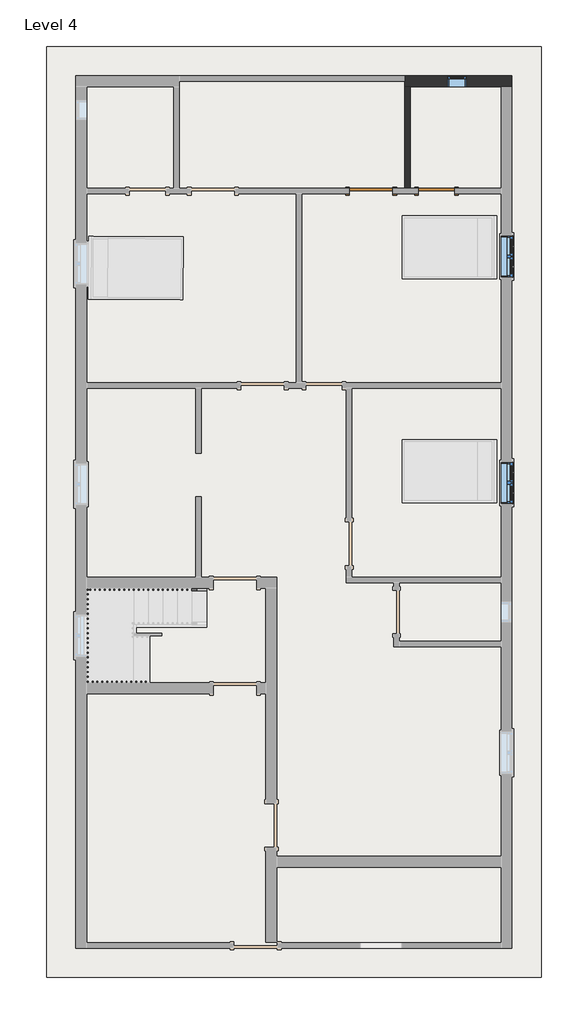
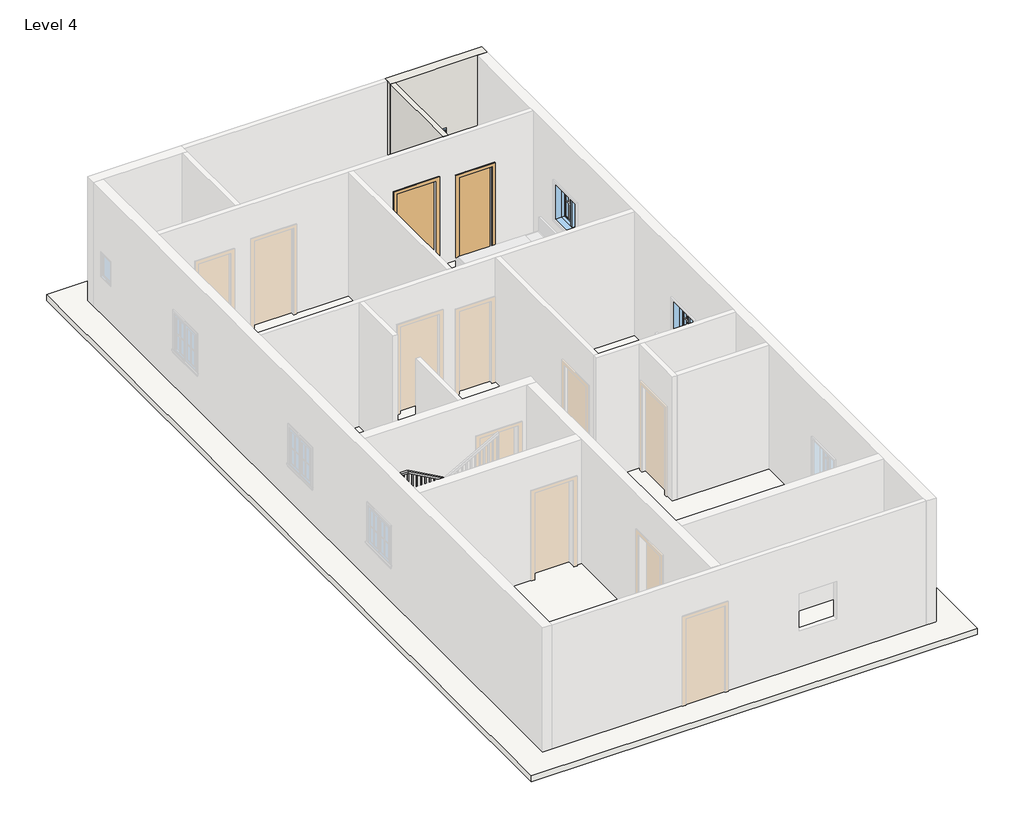
# One storey, part 2 of 3: 3 windows, 2 doors, 2 walls, 1 railing, 1 roof.
"""IFC4 building model written with IfcOpenShell, lengths in millimetres."""

from ifc_helpers import new_model, si_unit, frame, origin, place, context, project, spatial, polyline, outline, extrude, faceted_brep, transform, mapped, element, save
from components import door_f2b275c1, door_e5f9f3c4, window_aa618e30, window_339605e1

model = new_model("IFC4")

# Units and contexts
model_context = context("Model", 3, world=origin())
ifc_project = project(units=[si_unit("LENGTHUNIT", "METRE", prefix="MILLI")], contexts=[model_context])

# Site, building, storey
site = spatial("IfcSite", under=ifc_project)
building = spatial("IfcBuilding", under=site)
storey = spatial("IfcBuildingStorey", under=building, Name="Level 4", Elevation=6400.8)

# Doors
placement = place(None, origin())
door_shape = door_f2b275c1(model_context)
element("IfcDoor", 1, ObjectType="Single-Flush : 30\" x 80\"", at=placement, inside=storey, context=model_context, shape_type="MappedRepresentation", body=[
    mapped(door_shape, transform((1735.6084916, 8007.7072267, 6400.8), x_axis=(-1.0, 0.0, 0.0), y_axis=(0.0, -1.0, 0.0), z_axis=(0.0, 0.0, 1.0))),
])
door_2_shape = door_e5f9f3c4(model_context)
element("IfcDoor", 2, ObjectType="Single-Flush : 36\" x 84\"", at=placement, inside=storey, context=model_context, shape_type="MappedRepresentation", body=[
    mapped(door_2_shape, transform((364.0084916, 8007.7072267, 6400.8), x_axis=(1.0, 0.0, 0.0), y_axis=(0.0, 1.0, 0.0), z_axis=(0.0, 0.0, 1.0))),
])

# Railing
element("IfcRailing", 3, ObjectType="Handrail - Rectangular", at=placement, inside=storey, context=model_context, shape_type="SolidModel", body=[
    faceted_brep([(-3084.0415084, -367.9427733, 7484.5333333), (-3084.0415084, -367.9427733, 7426.420221), (-3084.0415084, -317.1427733, 7426.420221), (-3084.0415084, -317.1427733, 7484.5333333), (-4608.0415084, -367.9427733, 8331.2), (-4621.2051106, -367.9427733, 8280.4), (-4621.2051106, -317.1427733, 8280.4), (-4608.0415084, -317.1427733, 8331.2), (-5547.8415084, -367.9427733, 8331.2), (-5547.8415084, -367.9427733, 8280.4), (-5598.6415084, -317.1427733, 8280.4), (-5598.6415084, -317.1427733, 8331.2), (-5547.8415084, -2247.5427733, 8331.2), (-5547.8415084, -2247.5427733, 8280.4), (-5598.6415084, -2298.3427733, 8280.4), (-5598.6415084, -2298.3427733, 8331.2), (-4912.8415084, -2247.5427733, 8331.2), (-4899.6779062, -2247.5427733, 8280.4), (-4899.6779062, -2298.3427733, 8280.4), (-4912.8415084, -2298.3427733, 8331.2), (-3084.0415084, -2247.5427733, 9347.2), (-3084.0415084, -2298.3427733, 9347.2), (-3084.0415084, -2298.3427733, 9289.0868876), (-3084.0415084, -2247.5427733, 9289.0868876)], [[[0, 1, 2, 3]], [[1, 0, 4, 5]], [[2, 1, 5, 6]], [[3, 2, 6, 7]], [[0, 3, 7, 4]], [[5, 4, 8, 9]], [[6, 5, 9, 10]], [[7, 6, 10, 11]], [[4, 7, 11, 8]], [[9, 8, 12, 13]], [[10, 9, 13, 14]], [[11, 10, 14, 15]], [[8, 11, 15, 12]], [[13, 12, 16, 17]], [[14, 13, 17, 18]], [[15, 14, 18, 19]], [[12, 15, 19, 16]], [[20, 21, 22, 23]], [[17, 16, 20, 23]], [[18, 17, 23, 22]], [[19, 18, 22, 21]], [[16, 19, 21, 20]]]),
    extrude(outline(polyline([(9266.1563321, -3125.3165084), (9255.5729988, -3144.3665084), (8263.4666667, -3144.3665084), (8263.4666667, -3125.3165084), (9266.1563321, -3125.3165084)])), frame((0.0, -2282.4677733, 0.0), z_axis=(0.0, 1.0, 0.0), x_axis=(0.0, 0.0, 1.0)), (0.0, 0.0, 1.0), 19.05),
    extrude(outline(polyline([(9209.7118876, -3226.9165084), (9199.1285543, -3245.9665084), (8263.4666667, -3245.9665084), (8263.4666667, -3226.9165084), (9209.7118876, -3226.9165084)])), frame((0.0, -2282.4677733, 0.0), z_axis=(0.0, 1.0, 0.0), x_axis=(0.0, 0.0, 1.0)), (0.0, 0.0, 1.0), 19.05),
    extrude(outline(polyline([(9153.2674432, -3328.5165084), (9142.6841099, -3347.5665084), (8263.4666667, -3347.5665084), (8263.4666667, -3328.5165084), (9153.2674432, -3328.5165084)])), frame((0.0, -2282.4677733, 0.0), z_axis=(0.0, 1.0, 0.0), x_axis=(0.0, 0.0, 1.0)), (0.0, 0.0, 1.0), 19.05),
    extrude(outline(polyline([(9096.8229988, -3430.1165084), (9086.2396654, -3449.1665084), (8094.1333333, -3449.1665084), (8094.1333333, -3430.1165084), (9096.8229988, -3430.1165084)])), frame((0.0, -2282.4677733, 0.0), z_axis=(0.0, 1.0, 0.0), x_axis=(0.0, 0.0, 1.0)), (0.0, 0.0, 1.0), 19.05),
    extrude(outline(polyline([(9040.3785543, -3531.7165084), (9029.795221, -3550.7665084), (8094.1333333, -3550.7665084), (8094.1333333, -3531.7165084), (9040.3785543, -3531.7165084)])), frame((0.0, -2282.4677733, 0.0), z_axis=(0.0, 1.0, 0.0), x_axis=(0.0, 0.0, 1.0)), (0.0, 0.0, 1.0), 19.05),
    extrude(outline(polyline([(8983.9341099, -3633.3165084), (8973.3507765, -3652.3665084), (8094.1333333, -3652.3665084), (8094.1333333, -3633.3165084), (8983.9341099, -3633.3165084)])), frame((0.0, -2282.4677733, 0.0), z_axis=(0.0, 1.0, 0.0), x_axis=(0.0, 0.0, 1.0)), (0.0, 0.0, 1.0), 19.05),
    extrude(outline(polyline([(8927.4896654, -3734.9165084), (8916.9063321, -3753.9665084), (7924.8, -3753.9665084), (7924.8, -3734.9165084), (8927.4896654, -3734.9165084)])), frame((0.0, -2282.4677733, 0.0), z_axis=(0.0, 1.0, 0.0), x_axis=(0.0, 0.0, 1.0)), (0.0, 0.0, 1.0), 19.05),
    extrude(outline(polyline([(8871.045221, -3836.5165084), (8860.4618876, -3855.5665084), (7924.8, -3855.5665084), (7924.8, -3836.5165084), (8871.045221, -3836.5165084)])), frame((0.0, -2282.4677733, 0.0), z_axis=(0.0, 1.0, 0.0), x_axis=(0.0, 0.0, 1.0)), (0.0, 0.0, 1.0), 19.05),
    extrude(outline(polyline([(8814.6007765, -3938.1165084), (8804.0174432, -3957.1665084), (7924.8, -3957.1665084), (7924.8, -3938.1165084), (8814.6007765, -3938.1165084)])), frame((0.0, -2282.4677733, 0.0), z_axis=(0.0, 1.0, 0.0), x_axis=(0.0, 0.0, 1.0)), (0.0, 0.0, 1.0), 19.05),
    extrude(outline(polyline([(8758.1563321, -4039.7165084), (8747.5729988, -4058.7665084), (7755.4666667, -4058.7665084), (7755.4666667, -4039.7165084), (8758.1563321, -4039.7165084)])), frame((0.0, -2282.4677733, 0.0), z_axis=(0.0, 1.0, 0.0), x_axis=(0.0, 0.0, 1.0)), (0.0, 0.0, 1.0), 19.05),
    extrude(outline(polyline([(8701.7118876, -4141.3165084), (8691.1285543, -4160.3665084), (7755.4666667, -4160.3665084), (7755.4666667, -4141.3165084), (8701.7118876, -4141.3165084)])), frame((0.0, -2282.4677733, 0.0), z_axis=(0.0, 1.0, 0.0), x_axis=(0.0, 0.0, 1.0)), (0.0, 0.0, 1.0), 19.05),
    extrude(outline(polyline([(8645.2674432, -4242.9165084), (8634.6841099, -4261.9665084), (7755.4666667, -4261.9665084), (7755.4666667, -4242.9165084), (8645.2674432, -4242.9165084)])), frame((0.0, -2282.4677733, 0.0), z_axis=(0.0, 1.0, 0.0), x_axis=(0.0, 0.0, 1.0)), (0.0, 0.0, 1.0), 19.05),
    extrude(outline(polyline([(8588.8229988, -4344.5165084), (8578.2396654, -4363.5665084), (7586.1333333, -4363.5665084), (7586.1333333, -4344.5165084), (8588.8229988, -4344.5165084)])), frame((0.0, -2282.4677733, 0.0), z_axis=(0.0, 1.0, 0.0), x_axis=(0.0, 0.0, 1.0)), (0.0, 0.0, 1.0), 19.05),
    extrude(outline(polyline([(8532.3785543, -4446.1165084), (8521.795221, -4465.1665084), (7586.1333333, -4465.1665084), (7586.1333333, -4446.1165084), (8532.3785543, -4446.1165084)])), frame((0.0, -2282.4677733, 0.0), z_axis=(0.0, 1.0, 0.0), x_axis=(0.0, 0.0, 1.0)), (0.0, 0.0, 1.0), 19.05),
    extrude(outline(polyline([(8475.9341099, -4547.7165084), (8465.3507765, -4566.7665084), (7586.1333333, -4566.7665084), (7586.1333333, -4547.7165084), (8475.9341099, -4547.7165084)])), frame((0.0, -2282.4677733, 0.0), z_axis=(0.0, 1.0, 0.0), x_axis=(0.0, 0.0, 1.0)), (0.0, 0.0, 1.0), 19.05),
    extrude(outline(polyline([(8419.4896654, -4649.3165084), (8408.9063321, -4668.3665084), (7416.8, -4668.3665084), (7416.8, -4649.3165084), (8419.4896654, -4649.3165084)])), frame((0.0, -2282.4677733, 0.0), z_axis=(0.0, 1.0, 0.0), x_axis=(0.0, 0.0, 1.0)), (0.0, 0.0, 1.0), 19.05),
    extrude(outline(polyline([(8363.045221, -4750.9165084), (8352.4618876, -4769.9665084), (7416.8, -4769.9665084), (7416.8, -4750.9165084), (8363.045221, -4750.9165084)])), frame((0.0, -2282.4677733, 0.0), z_axis=(0.0, 1.0, 0.0), x_axis=(0.0, 0.0, 1.0)), (0.0, 0.0, 1.0), 19.05),
    extrude(outline(polyline([(8306.6007765, -4852.5165084), (8296.0174432, -4871.5665084), (7416.8, -4871.5665084), (7416.8, -4852.5165084), (8306.6007765, -4852.5165084)])), frame((0.0, -2282.4677733, 0.0), z_axis=(0.0, 1.0, 0.0), x_axis=(0.0, 0.0, 1.0)), (0.0, 0.0, 1.0), 19.05),
    extrude(outline(polyline([(-4973.1665084, -2282.4677733), (-4973.1665084, -2263.4177733), (-4954.1165084, -2263.4177733), (-4954.1165084, -2282.4677733), (-4973.1665084, -2282.4677733)])), frame((0.0, 0.0, 7416.8), z_axis=(0.0, 0.0, 1.0), x_axis=(1.0, 0.0, 0.0)), (0.0, 0.0, 1.0), 863.6),
    extrude(outline(polyline([(-5074.7665084, -2282.4677733), (-5074.7665084, -2263.4177733), (-5055.7165084, -2263.4177733), (-5055.7165084, -2282.4677733), (-5074.7665084, -2282.4677733)])), frame((0.0, 0.0, 7416.8), z_axis=(0.0, 0.0, 1.0), x_axis=(1.0, 0.0, 0.0)), (0.0, 0.0, 1.0), 863.6),
    extrude(outline(polyline([(-5176.3665084, -2282.4677733), (-5176.3665084, -2263.4177733), (-5157.3165084, -2263.4177733), (-5157.3165084, -2282.4677733), (-5176.3665084, -2282.4677733)])), frame((0.0, 0.0, 7416.8), z_axis=(0.0, 0.0, 1.0), x_axis=(1.0, 0.0, 0.0)), (0.0, 0.0, 1.0), 863.6),
    extrude(outline(polyline([(-5277.9665084, -2282.4677733), (-5277.9665084, -2263.4177733), (-5258.9165084, -2263.4177733), (-5258.9165084, -2282.4677733), (-5277.9665084, -2282.4677733)])), frame((0.0, 0.0, 7416.8), z_axis=(0.0, 0.0, 1.0), x_axis=(1.0, 0.0, 0.0)), (0.0, 0.0, 1.0), 863.6),
    extrude(outline(polyline([(-5379.5665084, -2282.4677733), (-5379.5665084, -2263.4177733), (-5360.5165084, -2263.4177733), (-5360.5165084, -2282.4677733), (-5379.5665084, -2282.4677733)])), frame((0.0, 0.0, 7416.8), z_axis=(0.0, 0.0, 1.0), x_axis=(1.0, 0.0, 0.0)), (0.0, 0.0, 1.0), 863.6),
    extrude(outline(polyline([(-5481.1665084, -2282.4677733), (-5481.1665084, -2263.4177733), (-5462.1165084, -2263.4177733), (-5462.1165084, -2282.4677733), (-5481.1665084, -2282.4677733)])), frame((0.0, 0.0, 7416.8), z_axis=(0.0, 0.0, 1.0), x_axis=(1.0, 0.0, 0.0)), (0.0, 0.0, 1.0), 863.6),
    extrude(outline(polyline([(-5582.7665084, -2161.8177733), (-5563.7165084, -2161.8177733), (-5563.7165084, -2180.8677733), (-5582.7665084, -2180.8677733), (-5582.7665084, -2161.8177733)])), frame((0.0, 0.0, 7416.8), z_axis=(0.0, 0.0, 1.0), x_axis=(1.0, 0.0, 0.0)), (0.0, 0.0, 1.0), 863.6),
    extrude(outline(polyline([(-5582.7665084, -2060.2177733), (-5563.7165084, -2060.2177733), (-5563.7165084, -2079.2677733), (-5582.7665084, -2079.2677733), (-5582.7665084, -2060.2177733)])), frame((0.0, 0.0, 7416.8), z_axis=(0.0, 0.0, 1.0), x_axis=(1.0, 0.0, 0.0)), (0.0, 0.0, 1.0), 863.6),
    extrude(outline(polyline([(-5582.7665084, -1958.6177733), (-5563.7165084, -1958.6177733), (-5563.7165084, -1977.6677733), (-5582.7665084, -1977.6677733), (-5582.7665084, -1958.6177733)])), frame((0.0, 0.0, 7416.8), z_axis=(0.0, 0.0, 1.0), x_axis=(1.0, 0.0, 0.0)), (0.0, 0.0, 1.0), 863.6),
    extrude(outline(polyline([(-5582.7665084, -1857.0177733), (-5563.7165084, -1857.0177733), (-5563.7165084, -1876.0677733), (-5582.7665084, -1876.0677733), (-5582.7665084, -1857.0177733)])), frame((0.0, 0.0, 7416.8), z_axis=(0.0, 0.0, 1.0), x_axis=(1.0, 0.0, 0.0)), (0.0, 0.0, 1.0), 863.6),
    extrude(outline(polyline([(-5582.7665084, -1755.4177733), (-5563.7165084, -1755.4177733), (-5563.7165084, -1774.4677733), (-5582.7665084, -1774.4677733), (-5582.7665084, -1755.4177733)])), frame((0.0, 0.0, 7416.8), z_axis=(0.0, 0.0, 1.0), x_axis=(1.0, 0.0, 0.0)), (0.0, 0.0, 1.0), 863.6),
    extrude(outline(polyline([(-5582.7665084, -1653.8177733), (-5563.7165084, -1653.8177733), (-5563.7165084, -1672.8677733), (-5582.7665084, -1672.8677733), (-5582.7665084, -1653.8177733)])), frame((0.0, 0.0, 7416.8), z_axis=(0.0, 0.0, 1.0), x_axis=(1.0, 0.0, 0.0)), (0.0, 0.0, 1.0), 863.6),
    extrude(outline(polyline([(-5582.7665084, -1552.2177733), (-5563.7165084, -1552.2177733), (-5563.7165084, -1571.2677733), (-5582.7665084, -1571.2677733), (-5582.7665084, -1552.2177733)])), frame((0.0, 0.0, 7416.8), z_axis=(0.0, 0.0, 1.0), x_axis=(1.0, 0.0, 0.0)), (0.0, 0.0, 1.0), 863.6),
    extrude(outline(polyline([(-5582.7665084, -1450.6177733), (-5563.7165084, -1450.6177733), (-5563.7165084, -1469.6677733), (-5582.7665084, -1469.6677733), (-5582.7665084, -1450.6177733)])), frame((0.0, 0.0, 7416.8), z_axis=(0.0, 0.0, 1.0), x_axis=(1.0, 0.0, 0.0)), (0.0, 0.0, 1.0), 863.6),
    extrude(outline(polyline([(-5582.7665084, -1349.0177733), (-5563.7165084, -1349.0177733), (-5563.7165084, -1368.0677733), (-5582.7665084, -1368.0677733), (-5582.7665084, -1349.0177733)])), frame((0.0, 0.0, 7416.8), z_axis=(0.0, 0.0, 1.0), x_axis=(1.0, 0.0, 0.0)), (0.0, 0.0, 1.0), 863.6),
    extrude(outline(polyline([(-5582.7665084, -1247.4177733), (-5563.7165084, -1247.4177733), (-5563.7165084, -1266.4677733), (-5582.7665084, -1266.4677733), (-5582.7665084, -1247.4177733)])), frame((0.0, 0.0, 7416.8), z_axis=(0.0, 0.0, 1.0), x_axis=(1.0, 0.0, 0.0)), (0.0, 0.0, 1.0), 863.6),
    extrude(outline(polyline([(-5582.7665084, -1145.8177733), (-5563.7165084, -1145.8177733), (-5563.7165084, -1164.8677733), (-5582.7665084, -1164.8677733), (-5582.7665084, -1145.8177733)])), frame((0.0, 0.0, 7416.8), z_axis=(0.0, 0.0, 1.0), x_axis=(1.0, 0.0, 0.0)), (0.0, 0.0, 1.0), 863.6),
    extrude(outline(polyline([(-5582.7665084, -1044.2177733), (-5563.7165084, -1044.2177733), (-5563.7165084, -1063.2677733), (-5582.7665084, -1063.2677733), (-5582.7665084, -1044.2177733)])), frame((0.0, 0.0, 7416.8), z_axis=(0.0, 0.0, 1.0), x_axis=(1.0, 0.0, 0.0)), (0.0, 0.0, 1.0), 863.6),
    extrude(outline(polyline([(-5582.7665084, -942.6177733), (-5563.7165084, -942.6177733), (-5563.7165084, -961.6677733), (-5582.7665084, -961.6677733), (-5582.7665084, -942.6177733)])), frame((0.0, 0.0, 7416.8), z_axis=(0.0, 0.0, 1.0), x_axis=(1.0, 0.0, 0.0)), (0.0, 0.0, 1.0), 863.6),
    extrude(outline(polyline([(-5582.7665084, -841.0177733), (-5563.7165084, -841.0177733), (-5563.7165084, -860.0677733), (-5582.7665084, -860.0677733), (-5582.7665084, -841.0177733)])), frame((0.0, 0.0, 7416.8), z_axis=(0.0, 0.0, 1.0), x_axis=(1.0, 0.0, 0.0)), (0.0, 0.0, 1.0), 863.6),
    extrude(outline(polyline([(-5582.7665084, -739.4177733), (-5563.7165084, -739.4177733), (-5563.7165084, -758.4677733), (-5582.7665084, -758.4677733), (-5582.7665084, -739.4177733)])), frame((0.0, 0.0, 7416.8), z_axis=(0.0, 0.0, 1.0), x_axis=(1.0, 0.0, 0.0)), (0.0, 0.0, 1.0), 863.6),
    extrude(outline(polyline([(-5582.7665084, -637.8177733), (-5563.7165084, -637.8177733), (-5563.7165084, -656.8677733), (-5582.7665084, -656.8677733), (-5582.7665084, -637.8177733)])), frame((0.0, 0.0, 7416.8), z_axis=(0.0, 0.0, 1.0), x_axis=(1.0, 0.0, 0.0)), (0.0, 0.0, 1.0), 863.6),
    extrude(outline(polyline([(-5582.7665084, -536.2177733), (-5563.7165084, -536.2177733), (-5563.7165084, -555.2677733), (-5582.7665084, -555.2677733), (-5582.7665084, -536.2177733)])), frame((0.0, 0.0, 7416.8), z_axis=(0.0, 0.0, 1.0), x_axis=(1.0, 0.0, 0.0)), (0.0, 0.0, 1.0), 863.6),
    extrude(outline(polyline([(-5582.7665084, -434.6177733), (-5563.7165084, -434.6177733), (-5563.7165084, -453.6677733), (-5582.7665084, -453.6677733), (-5582.7665084, -434.6177733)])), frame((0.0, 0.0, 7416.8), z_axis=(0.0, 0.0, 1.0), x_axis=(1.0, 0.0, 0.0)), (0.0, 0.0, 1.0), 863.6),
    extrude(outline(polyline([(-5512.9165084, -333.0177733), (-5512.9165084, -352.0677733), (-5531.9665084, -352.0677733), (-5531.9665084, -333.0177733), (-5512.9165084, -333.0177733)])), frame((0.0, 0.0, 7416.8), z_axis=(0.0, 0.0, 1.0), x_axis=(1.0, 0.0, 0.0)), (0.0, 0.0, 1.0), 863.6),
    extrude(outline(polyline([(-5411.3165084, -333.0177733), (-5411.3165084, -352.0677733), (-5430.3665084, -352.0677733), (-5430.3665084, -333.0177733), (-5411.3165084, -333.0177733)])), frame((0.0, 0.0, 7416.8), z_axis=(0.0, 0.0, 1.0), x_axis=(1.0, 0.0, 0.0)), (0.0, 0.0, 1.0), 863.6),
    extrude(outline(polyline([(-5309.7165084, -333.0177733), (-5309.7165084, -352.0677733), (-5328.7665084, -352.0677733), (-5328.7665084, -333.0177733), (-5309.7165084, -333.0177733)])), frame((0.0, 0.0, 7416.8), z_axis=(0.0, 0.0, 1.0), x_axis=(1.0, 0.0, 0.0)), (0.0, 0.0, 1.0), 863.6),
    extrude(outline(polyline([(-5208.1165084, -333.0177733), (-5208.1165084, -352.0677733), (-5227.1665084, -352.0677733), (-5227.1665084, -333.0177733), (-5208.1165084, -333.0177733)])), frame((0.0, 0.0, 7416.8), z_axis=(0.0, 0.0, 1.0), x_axis=(1.0, 0.0, 0.0)), (0.0, 0.0, 1.0), 863.6),
    extrude(outline(polyline([(-5106.5165084, -333.0177733), (-5106.5165084, -352.0677733), (-5125.5665084, -352.0677733), (-5125.5665084, -333.0177733), (-5106.5165084, -333.0177733)])), frame((0.0, 0.0, 7416.8), z_axis=(0.0, 0.0, 1.0), x_axis=(1.0, 0.0, 0.0)), (0.0, 0.0, 1.0), 863.6),
    extrude(outline(polyline([(-5004.9165084, -333.0177733), (-5004.9165084, -352.0677733), (-5023.9665084, -352.0677733), (-5023.9665084, -333.0177733), (-5004.9165084, -333.0177733)])), frame((0.0, 0.0, 7416.8), z_axis=(0.0, 0.0, 1.0), x_axis=(1.0, 0.0, 0.0)), (0.0, 0.0, 1.0), 863.6),
    extrude(outline(polyline([(-4903.3165084, -333.0177733), (-4903.3165084, -352.0677733), (-4922.3665084, -352.0677733), (-4922.3665084, -333.0177733), (-4903.3165084, -333.0177733)])), frame((0.0, 0.0, 7416.8), z_axis=(0.0, 0.0, 1.0), x_axis=(1.0, 0.0, 0.0)), (0.0, 0.0, 1.0), 863.6),
    extrude(outline(polyline([(-4801.7165084, -333.0177733), (-4801.7165084, -352.0677733), (-4820.7665084, -352.0677733), (-4820.7665084, -333.0177733), (-4801.7165084, -333.0177733)])), frame((0.0, 0.0, 7416.8), z_axis=(0.0, 0.0, 1.0), x_axis=(1.0, 0.0, 0.0)), (0.0, 0.0, 1.0), 863.6),
    extrude(outline(polyline([(-4700.1165084, -333.0177733), (-4700.1165084, -352.0677733), (-4719.1665084, -352.0677733), (-4719.1665084, -333.0177733), (-4700.1165084, -333.0177733)])), frame((0.0, 0.0, 7416.8), z_axis=(0.0, 0.0, 1.0), x_axis=(1.0, 0.0, 0.0)), (0.0, 0.0, 1.0), 863.6),
    extrude(outline(polyline([(8267.795221, -4598.5165084), (8278.3785543, -4617.5665084), (7416.8, -4617.5665084), (7416.8, -4598.5165084), (8267.795221, -4598.5165084)])), frame((0.0, -352.0677733, 0.0), z_axis=(0.0, 1.0, 0.0), x_axis=(0.0, 0.0, 1.0)), (0.0, 0.0, 1.0), 19.05),
    extrude(outline(polyline([(8211.3507765, -4496.9165084), (8221.9341099, -4515.9665084), (7247.4666667, -4515.9665084), (7247.4666667, -4496.9165084), (8211.3507765, -4496.9165084)])), frame((0.0, -352.0677733, 0.0), z_axis=(0.0, 1.0, 0.0), x_axis=(0.0, 0.0, 1.0)), (0.0, 0.0, 1.0), 19.05),
    extrude(outline(polyline([(8154.9063321, -4395.3165084), (8165.4896654, -4414.3665084), (7247.4666667, -4414.3665084), (7247.4666667, -4395.3165084), (8154.9063321, -4395.3165084)])), frame((0.0, -352.0677733, 0.0), z_axis=(0.0, 1.0, 0.0), x_axis=(0.0, 0.0, 1.0)), (0.0, 0.0, 1.0), 19.05),
    extrude(outline(polyline([(8098.4618876, -4293.7165084), (8109.045221, -4312.7665084), (7247.4666667, -4312.7665084), (7247.4666667, -4293.7165084), (8098.4618876, -4293.7165084)])), frame((0.0, -352.0677733, 0.0), z_axis=(0.0, 1.0, 0.0), x_axis=(0.0, 0.0, 1.0)), (0.0, 0.0, 1.0), 19.05),
    extrude(outline(polyline([(8042.0174432, -4192.1165084), (8052.6007765, -4211.1665084), (7078.1333333, -4211.1665084), (7078.1333333, -4192.1165084), (8042.0174432, -4192.1165084)])), frame((0.0, -352.0677733, 0.0), z_axis=(0.0, 1.0, 0.0), x_axis=(0.0, 0.0, 1.0)), (0.0, 0.0, 1.0), 19.05),
    extrude(outline(polyline([(7985.5729988, -4090.5165084), (7996.1563321, -4109.5665084), (7078.1333333, -4109.5665084), (7078.1333333, -4090.5165084), (7985.5729988, -4090.5165084)])), frame((0.0, -352.0677733, 0.0), z_axis=(0.0, 1.0, 0.0), x_axis=(0.0, 0.0, 1.0)), (0.0, 0.0, 1.0), 19.05),
    extrude(outline(polyline([(7929.1285543, -3988.9165084), (7939.7118876, -4007.9665084), (7078.1333333, -4007.9665084), (7078.1333333, -3988.9165084), (7929.1285543, -3988.9165084)])), frame((0.0, -352.0677733, 0.0), z_axis=(0.0, 1.0, 0.0), x_axis=(0.0, 0.0, 1.0)), (0.0, 0.0, 1.0), 19.05),
    extrude(outline(polyline([(7872.6841099, -3887.3165084), (7883.2674432, -3906.3665084), (6908.8, -3906.3665084), (6908.8, -3887.3165084), (7872.6841099, -3887.3165084)])), frame((0.0, -352.0677733, 0.0), z_axis=(0.0, 1.0, 0.0), x_axis=(0.0, 0.0, 1.0)), (0.0, 0.0, 1.0), 19.05),
    extrude(outline(polyline([(7816.2396654, -3785.7165084), (7826.8229988, -3804.7665084), (6908.8, -3804.7665084), (6908.8, -3785.7165084), (7816.2396654, -3785.7165084)])), frame((0.0, -352.0677733, 0.0), z_axis=(0.0, 1.0, 0.0), x_axis=(0.0, 0.0, 1.0)), (0.0, 0.0, 1.0), 19.05),
    extrude(outline(polyline([(7759.795221, -3684.1165084), (7770.3785543, -3703.1665084), (6908.8, -3703.1665084), (6908.8, -3684.1165084), (7759.795221, -3684.1165084)])), frame((0.0, -352.0677733, 0.0), z_axis=(0.0, 1.0, 0.0), x_axis=(0.0, 0.0, 1.0)), (0.0, 0.0, 1.0), 19.05),
    extrude(outline(polyline([(7703.3507765, -3582.5165084), (7713.9341099, -3601.5665084), (6739.4666667, -3601.5665084), (6739.4666667, -3582.5165084), (7703.3507765, -3582.5165084)])), frame((0.0, -352.0677733, 0.0), z_axis=(0.0, 1.0, 0.0), x_axis=(0.0, 0.0, 1.0)), (0.0, 0.0, 1.0), 19.05),
    extrude(outline(polyline([(7646.9063321, -3480.9165084), (7657.4896654, -3499.9665084), (6739.4666667, -3499.9665084), (6739.4666667, -3480.9165084), (7646.9063321, -3480.9165084)])), frame((0.0, -352.0677733, 0.0), z_axis=(0.0, 1.0, 0.0), x_axis=(0.0, 0.0, 1.0)), (0.0, 0.0, 1.0), 19.05),
    extrude(outline(polyline([(7590.4618876, -3379.3165084), (7601.045221, -3398.3665084), (6739.4666667, -3398.3665084), (6739.4666667, -3379.3165084), (7590.4618876, -3379.3165084)])), frame((0.0, -352.0677733, 0.0), z_axis=(0.0, 1.0, 0.0), x_axis=(0.0, 0.0, 1.0)), (0.0, 0.0, 1.0), 19.05),
    extrude(outline(polyline([(7534.0174432, -3277.7165084), (7544.6007765, -3296.7665084), (6570.1333333, -3296.7665084), (6570.1333333, -3277.7165084), (7534.0174432, -3277.7165084)])), frame((0.0, -352.0677733, 0.0), z_axis=(0.0, 1.0, 0.0), x_axis=(0.0, 0.0, 1.0)), (0.0, 0.0, 1.0), 19.05),
    extrude(outline(polyline([(7477.5729988, -3176.1165084), (7488.1563321, -3195.1665084), (6570.1333333, -3195.1665084), (6570.1333333, -3176.1165084), (7477.5729988, -3176.1165084)])), frame((0.0, -352.0677733, 0.0), z_axis=(0.0, 1.0, 0.0), x_axis=(0.0, 0.0, 1.0)), (0.0, 0.0, 1.0), 19.05),
    extrude(outline(polyline([(-5582.7665084, -2263.4177733), (-5563.7165084, -2263.4177733), (-5563.7165084, -2282.4677733), (-5582.7665084, -2282.4677733), (-5582.7665084, -2263.4177733)])), frame((0.0, 0.0, 7416.8), z_axis=(0.0, 0.0, 1.0), x_axis=(1.0, 0.0, 0.0)), (0.0, 0.0, 1.0), 863.6),
    extrude(outline(polyline([(-5563.7165084, -333.0177733), (-5563.7165084, -352.0677733), (-5582.7665084, -352.0677733), (-5582.7665084, -333.0177733), (-5563.7165084, -333.0177733)])), frame((0.0, 0.0, 7416.8), z_axis=(0.0, 0.0, 1.0), x_axis=(1.0, 0.0, 0.0)), (0.0, 0.0, 1.0), 863.6),
    extrude(outline(polyline([(9289.0868876, -3084.0415084), (9278.5035543, -3103.0915084), (8263.4666667, -3103.0915084), (8263.4666667, -3084.0415084), (9289.0868876, -3084.0415084)])), frame((0.0, -2282.4677733, 0.0), z_axis=(0.0, 1.0, 0.0), x_axis=(0.0, 0.0, 1.0)), (0.0, 0.0, 1.0), 19.05),
    extrude(outline(polyline([(7426.420221, -3084.0415084), (7437.0035543, -3103.0915084), (6570.1333333, -3103.0915084), (6570.1333333, -3084.0415084), (7426.420221, -3084.0415084)])), frame((0.0, -352.0677733, 0.0), z_axis=(0.0, 1.0, 0.0), x_axis=(0.0, 0.0, 1.0)), (0.0, 0.0, 1.0), 19.05),
])

# Roof
element("IfcRoof", 4, ObjectType="Generic - 12\"", at=placement, inside=storey, context=model_context, shape_type="SweptSolid", body=[
    extrude(outline(polyline([(-6436.8415084, 11036.6572267), (3926.3584916, 11036.6572267), (3926.3584916, -8470.5427733), (-6436.8415084, -8470.5427733), (-6436.8415084, 11036.6572267)])), frame((0.0, 0.0, 6248.4), z_axis=(0.0, 0.0, 1.0), x_axis=(1.0, 0.0, 0.0)), (0.0, 0.0, 1.0), 152.4),
])

# Walls
element("IfcWall", 5, ObjectType="WALL4.5\"", at=placement, inside=storey, context=model_context, shape_type="SweptSolid", body=[
    extrude(outline(polyline([(1068.8584916, 8064.8572267), (1068.8584916, 10198.4572267), (1183.1584916, 10198.4572267), (1183.1584916, 8064.8572267), (1068.8584916, 8064.8572267)])), frame((0.0, 0.0, 6400.8), z_axis=(0.0, 0.0, 1.0), x_axis=(1.0, 0.0, 0.0)), (0.0, 0.0, 1.0), 3048.0),
])
element("IfcWall", 6, ObjectType="WALL9\"", at=placement, inside=storey, context=model_context, shape_type="Brep", body=[
    faceted_brep([(1068.8584916, 10198.4572267, 6400.8), (1183.1584916, 10198.4572267, 6400.8), (3088.1584916, 10198.4572267, 6400.8), (3316.7584916, 10198.4572267, 6400.8), (3316.7584916, 10198.4572267, 9448.8), (3088.1584916, 10198.4572267, 9448.8), (1183.1584916, 10198.4572267, 9448.8), (1068.8584916, 10198.4572267, 9448.8), (2367.4334916, 10198.4572267, 7924.8), (2367.4334916, 10198.4572267, 7315.2), (1961.0334916, 10198.4572267, 7315.2), (1961.0334916, 10198.4572267, 7924.8), (1068.8584916, 10427.0572267, 6400.8), (1068.8584916, 10427.0572267, 9448.8), (3316.7584916, 10427.0572267, 9448.8), (3316.7584916, 10427.0572267, 6400.8), (2367.4334916, 10427.0572267, 7924.8), (1961.0334916, 10427.0572267, 7924.8), (1961.0334916, 10427.0572267, 7315.2), (2367.4334916, 10427.0572267, 7315.2), (1068.8584916, 10312.7572267, 6400.8), (1068.8584916, 10312.7572267, 9448.8)], [[[0, 1, 2, 3, 4, 5, 6, 7], [8, 9, 10, 11]], [[12, 13, 14, 15], [16, 17, 18, 19]], [[3, 2, 1, 0, 20, 12, 15]], [[4, 3, 15, 14]], [[0, 7, 21, 13, 12, 20]], [[9, 8, 16, 19]], [[10, 9, 19, 18]], [[11, 10, 18, 17]], [[8, 11, 17, 16]], [[7, 6, 5, 4, 14, 13, 21]]]),
])

# Windows
window_shape = window_aa618e30(model_context)
element("IfcWindow", 7, ObjectType="Fixed : 16\" x 24\"", at=placement, inside=storey, context=model_context, shape_type="MappedRepresentation", body=[
    mapped(window_shape, transform((2202.3334916, 10312.7572267, 6400.8), x_axis=(1.0, 0.0, 0.0), y_axis=(0.0, 1.0, 0.0), z_axis=(0.0, 0.0, 1.0))),
])
window_2_shape = window_339605e1(model_context)
element("IfcWindow", 8, ObjectType="Window-Casement-Double : 34\" x 36\"", at=placement, inside=storey, context=model_context, shape_type="MappedRepresentation", body=[
    mapped(window_2_shape, transform((3202.4584916, 6636.1072267, 6400.8), x_axis=(0.0, -1.0, 0.0), y_axis=(1.0, 0.0, 0.0), z_axis=(0.0, 0.0, 1.0))),
])
element("IfcWindow", 9, ObjectType="Window-Casement-Double : 34\" x 36\"", at=placement, inside=storey, context=model_context, shape_type="MappedRepresentation", body=[
    mapped(window_2_shape, transform((3202.4584916, 1892.6572267, 6400.8), x_axis=(0.0, -1.0, 0.0), y_axis=(1.0, 0.0, 0.0), z_axis=(0.0, 0.0, 1.0))),
])

save(model, "model.ifc")

# Revit data of these elements
# Type "Single-Flush : 30\" x 80\""
#   Type Mark = "5"
#   Construction Type Id = "MDOOR"
#   Assembly Code = "C1020"
#   Analytic Construction = "Metal"
#   Thickness = 0' - 2"
#   Heat Transfer Coefficient (U) = 0.651978 BTU/(h·ft²·°F)
#   Height = 6' - 8"
#   Trim Projection Ext = 0' - 1"
#   Trim Projection Int = 0' - 1"
#   Trim Width = 0' - 3"
#   Width = 2' - 6"
#   Define Thermal Properties by = 1
#   Define Thermal Properties by = 1
#   Door Material = Door - Panel
#   Frame Material = Door - Frame
#   Visual Light Transmittance = 0
#   Solar Heat Gain Coefficient = 0
#   Function = (empty or 0)
#   Wall Closure = (empty or 0)
# Type "Single-Flush : 36\" x 84\""
#   Type Mark = "1"
#   Construction Type Id = "MDOOR"
#   Assembly Code = "C1020"
#   Analytic Construction = "Metal"
#   Thickness = 0' - 2"
#   Heat Transfer Coefficient (U) = 0.651978 BTU/(h·ft²·°F)
#   Height = 7' - 0"
#   Trim Projection Ext = 0' - 1"
#   Trim Projection Int = 0' - 1"
#   Trim Width = 0' - 3"
#   Width = 3' - 0"
#   Define Thermal Properties by = 1
#   Define Thermal Properties by = 1
#   Door Material = Door - Panel
#   Frame Material = Door - Frame
#   Visual Light Transmittance = 0
#   Solar Heat Gain Coefficient = 0
#   Function = (empty or 0)
#   Wall Closure = (empty or 0)
# Type "Handrail - Rectangular"
#   Assembly Code = "C2010400"
#   built-in parameter 1008612 = 0.0416667 (stored number, unit not read)
#   built-in parameter 1008611 = 0.0416667 (stored number, unit not read)
#   built-in parameter 1008609 = 0.333333 (stored number, unit not read)
#   built-in parameter 1008604 = 0.166667 (stored number, unit not read)
#   built-in parameter 1008603 = 0.166667 (stored number, unit not read)
#   Railing Height = 3' - 0"
#   built-in parameter 1008630 = 2
#   built-in parameter 1008610 = 2
#   built-in parameter 1008618 = Baluster - Square : 3/4"
# Type "Generic - 12\""
#   Assembly Code = "B1020"
#   Layers, outside or top first: 0' - 6" no material (function 1)
# Type "WALL4.5\""
#   Assembly Code = "B2010"
#   Layers, outside or top first: 0' - 4 1/2" no material (function 1)
# Type "WALL9\""
#   Assembly Code = "B2010"
#   Layers, outside or top first: 0' - 9" no material (function 1)
# Type "Fixed : 16\" x 24\""
#   Type Mark = "4"
#   Construction Type Id = "GSP4R"
#   Assembly Code = "B2020100"
#   Analytic Construction = "1/8 in Pilkington single glazing"
#   Visual Light Transmittance = 0.9
#   Solar Heat Gain Coefficient = 0.78
#   Heat Transfer Coefficient (U) = 0.6496 BTU/(h·ft²·°F)
#   Height = 2' - 0"
#   Default Sill Height = 3' - 0"
#   Width = 1' - 4"
#   Window Inset = 0' - 0 3/4"
#   Define Thermal Properties by = 1
#   Define Thermal Properties by = 1
#   Glass Pane Material = Glass
#   Sash Material = Sash
#   Wall Closure = (empty or 0)
# Type "Window-Casement-Double : 34\" x 36\""
#   Type Mark = "14"
#   Fire Rating = "0.5h"
#   Assembly Code = "B2020100"
#   Analytic Construction = "Double glazing - domestic"
#   Frame Extension [instance default] = 0' - 0 1/4"
#   Window Inset [instance default] = 0' - 0"
#   Wall Thickness [instance default] = 0' - 6"
#   Interior Wall Closure [instance default] = 0' - 2 1/4"
#   Half Width = 1' - 5"
#   Visual Light Transmittance = 0.81
#   Thermal Resistance (R) = 1.8146 (h·ft²·°F)/BTU
#   Solar Heat Gain Coefficient = 0.76
#   Rough Width = 2' - 10 1/2"
#   Rough Height = 3' - 0 1/2"
#   Height = 3' - 0"
#   Heat Transfer Coefficient (U) = 0.5511 BTU/(h·ft²·°F)
#   Exterior Wall Closure [instance default] = 0' - 1 1/4"
#   Extension Jamb [instance default] = 0' - 2 1/4"
#   Default Sill Height = 3' - 0"
#   Width = 2' - 10"
#   Define Thermal Properties by = 0
#   Muntin Visibility = yes
#   Interior Trim Visibility [instance default] = yes
#   Exterior Trim Visibility [instance default] = yes
#   Extension Jamb Visibility [instance default] = yes
#   Interior Trim Material = Wood - Stained
#   Muntin Pattern = Muntin Pattern_2x2 : Muntin Pattern_2x2
#   Interior Trim = Trim-Window-Interior-Flat : Picture Frame
#   Interior Frame Material = Wood - Stained
#   Glass Panel Material = Glass
#   Exterior Trim Material = Clad - White
#   Exterior Trim = Trim-Window-Exterior-Flat : with Sill
#   Exterior Frame Material = Clad - White
#   Wall Closure = (empty or 0)
# Element 1 (IfcDoor, "Single-Flush : 30\" x 80\"")
#   Phase Created = New Construction
#   Materials on its faces: "Door - Frame", "Door - Panel"
# Element 2 (IfcDoor, "Single-Flush : 36\" x 84\"")
#   Phase Created = New Construction
#   Materials on its faces: "Door - Frame", "Door - Panel"
# Element 3 (IfcRailing, "Handrail - Rectangular")
#   Phase Created = New Construction
# Element 4 (IfcRoof, "Generic - 12\"")
#   built-in parameter 1001705 = 21 (stored number, unit not read)
#   built-in parameter 1001701 = -0.5 (stored number, unit not read)
#   built-in parameter 1001710 = 33615
#   Phase Created = New Construction
#   Materials on its faces: "Default Roof", "Wood Planks"
# Element 5 (IfcWall, "WALL4.5\"")
#   Top Offset = 0' - 0"
#   Base Offset = 0' - 0"
#   Unconnected Height = 10' - 0"
#   wall height = 10' - 0"
#   Phase Created = New Construction
#   Base Constraint = Level 4
#   Materials on its faces: "Default Wall", "Wood Planks"
# Element 6 (IfcWall, "WALL9\"")
#   Top Offset = 0' - 0"
#   Base Offset = 0' - 0"
#   Unconnected Height = 10' - 0"
#   wall height = 10' - 0"
#   Phase Created = New Construction
#   Base Constraint = Level 4
#   Materials on its faces: "Default Wall", "Wood Planks"
# Element 7 (IfcWindow, "Fixed : 16\" x 24\"")
#   Mark = "20"
#   Phase Created = New Construction
#   Materials on its faces: "Sash", "Glass"
# Element 8 (IfcWindow, "Window-Casement-Double : 34\" x 36\"")
#   Mark = "22"
#   Window Inset = 0' - 0"
#   Interior Wall Closure = 0' - 2 1/4"
#   Frame Extension = 0' - 0 1/4"
#   Exterior Wall Closure = 0' - 1 1/4"
#   Interior Trim Visibility = yes
#   Exterior Trim Visibility = yes
#   Phase Created = New Construction
#   Materials on its faces: "Wood - Stained", "Glass", "Clad - White"
# Element 9 (IfcWindow, "Window-Casement-Double : 34\" x 36\"")
#   Mark = "23"
#   Window Inset = 0' - 0"
#   Interior Wall Closure = 0' - 2 1/4"
#   Frame Extension = 0' - 0 1/4"
#   Exterior Wall Closure = 0' - 1 1/4"
#   Interior Trim Visibility = yes
#   Exterior Trim Visibility = yes
#   Phase Created = New Construction
#   Materials on its faces: "Wood - Stained", "Glass", "Clad - White"
# Materials
#   "Door - Panel": class "Wood", colour RGB 210 159 95, transparency 0, Cost = 0
#   "Door - Frame": colour RGB 118 70 51, transparency 0, Cost = 0
#   "Glass": class "Glass", colour RGB 0 128 192, transparency 0.75, Description = "Soda Lime Glass", Cost = 0
#   "Sash": class "Wood", colour RGB 224 178 126, transparency 0, Cost = 0
#   "Wood - Stained": class "Wood", colour RGB 224 178 126, transparency 0, Cost = 0
#   "Clad - White": class "Wood", colour RGB 242 242 238, transparency 0, Cost = 0
#   "Default Roof": colour RGB 88 101 114, transparency 0, Cost = 0
#   "Wood Planks": class "Wood", colour RGB 193 160 115, transparency 0, Description = "Physical material.", Cost = 0
#   "Default Wall": colour RGB 128 128 128, transparency 0, Cost = 0
